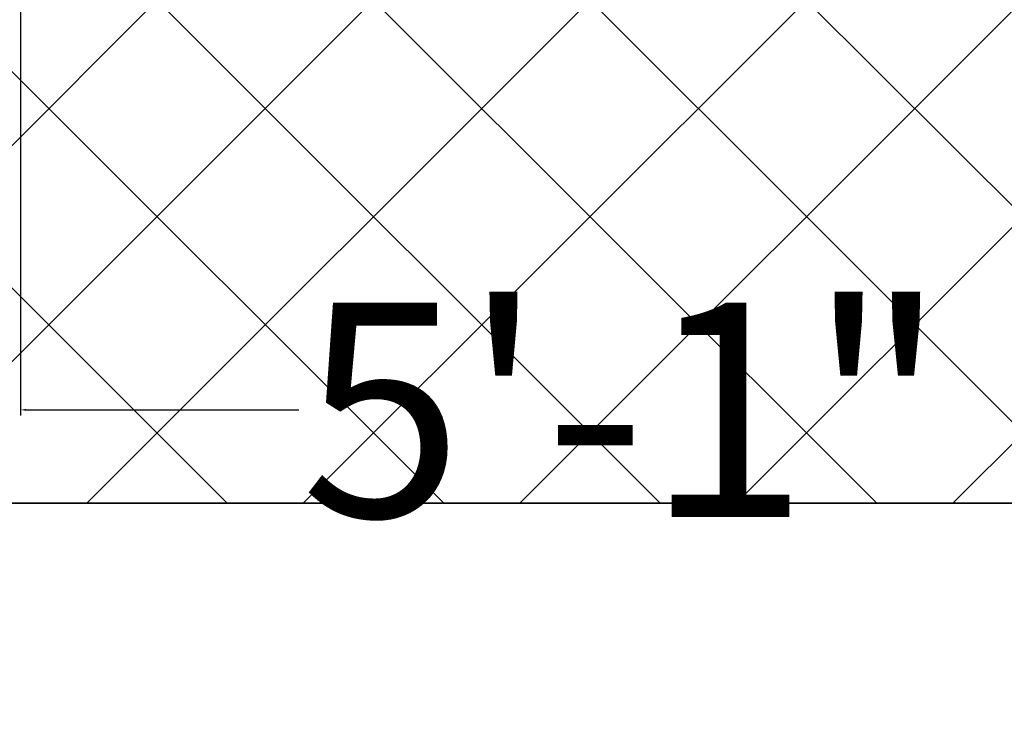
# Model space of a CAD drawing. Units: inches. Extents: x 2167 to 2589, y 1680 to 2489.
# Tile 2 of 38: x 2251 to 2283, y 1680 to 1703. Entities that reach past the tile are written whole.
import ezdxf

# ---------------------------------------------------------------- set-up
doc = ezdxf.new("R2010")
doc.units = ezdxf.units.IN
doc.header["$MEASUREMENT"] = 0
for name, color, linetype, lineweight in [('A-ANNO-DIMS', 2, 'Continuous', 18), ('C-PROP', 7, 'Continuous', 35), ('L-PVMT-PATT', 252, 'Continuous', 13)]:
    doc.layers.add(name, color=color, linetype=linetype, lineweight=lineweight)
doc.styles.get("Standard").update_dxf_attribs({"font": 'arial.ttf'})
doc.dimstyles.get("Standard").update_dxf_attribs({"dimtxt": 7, "dimasz": 0.18, "dimexe": 0.18, "dimexo": 0.0625, "dimgap": 0.09, "dimtad": 0, "dimtih": 1, "dimtoh": 1, "dimdec": 1, "dimzin": 0, "dimdsep": 46, "dimlunit": 3, "dimtxsty": 'Standard', "dimcen": 0.09, "dimadec": 0, "dimazin": 0, "dimtfac": 1, "dimtdec": 1, "dimtofl": 0, "dimtmove": 0, "dimatfit": 3, "dimfxl": 1, "dimtolj": 1, "dimtzin": 0, "dimarcsym": 0})

# ---------------------------------------------------------------- blocks, each defined once
blk = doc.blocks.new('*D46')
at = {"layer": 'A-ANNO-DIMS', "color": 0, "lineweight": -2, "transparency": 16777216}
for p, q in [((2251.218, 1709.362), (2251.218, 1690.565)), ((2312.254, 1709.362), (2312.254, 1690.565)), ((2251.398, 1690.745), (2260.312, 1690.745)), ((2312.074, 1690.745), (2303.16, 1690.745))]:
    blk.add_line(p, q, dxfattribs=at)
at = {"layer": 'A-ANNO-DIMS', "color": 0, "transparency": 16777216}
for points in [[(2251.398, 1690.775), (2251.398, 1690.715), (2251.218, 1690.745)], [(2312.074, 1690.775), (2312.074, 1690.715), (2312.254, 1690.745)]]:
    blk.add_solid(points, dxfattribs=at)
at = {"layer": 'Defpoints', "color": 0, "transparency": 16777216}
for p in [(2251.218, 1709.425), (2312.254, 1709.425), (2312.254, 1690.745)]:
    blk.add_point(p, dxfattribs=at)
at = {"layer": 'A-ANNO-DIMS', "color": 0, "transparency": 16777216, "insert": (2281.736, 1690.745), "char_height": 7, "attachment_point": 5}
blk.add_mtext('\\A1;5\'-1" TYP.', dxfattribs=at)

msp = doc.modelspace()

# ---------------------------------------------------------------- hatches: boundary and pattern name
at = {"layer": 'L-PVMT-PATT'}
h = msp.add_hatch(dxfattribs=at)
h.set_pattern_fill('ANSI37', color=256, scale=40)
h.paths.add_polyline_path([(2417.548, 1783.695), (2417.548, 1846.042), (2239.361, 1846.042), (2239.361, 1687.695), (2369.843, 1687.695), (2369.843, 1696.695), (2375.607, 1696.695), (2416.107, 1696.695), (2417.548, 1696.695)])

# ---------------------------------------------------------------- linework, layer by layer
at = {"layer": 'C-PROP'}
msp.add_line((2575.048, 1687.695), (2215.048, 1687.695), dxfattribs=at)

# ---------------------------------------------------------------- dimensions: what is measured, and where the dimension line sits
at = {"layer": 'A-ANNO-DIMS'}
dim = msp.add_linear_dim(base=(2312.254, 1690.745), p1=(2251.218, 1709.425), p2=(2312.254, 1709.425), text='<> TYP.', dimstyle='Standard', override={"dimdec": 1, "dimlfac": 1, "dimrnd": 0, "dimzin": 1, "dimdsep": 46, "dimlunit": 4, "dimfrac": 2}, dxfattribs=at)
dim.commit()
dim.dimension.update_dxf_attribs({"geometry": '*D46', "text_midpoint": (2281.736, 1690.745)})

doc.saveas('drawing.dxf')
